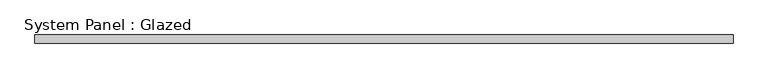
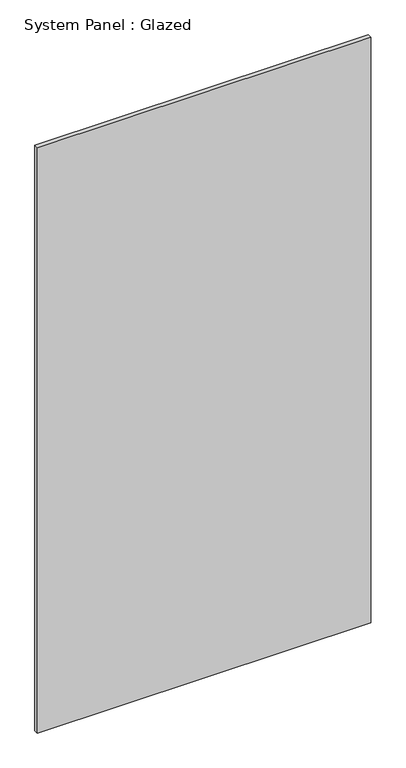
"""IFC4 building model written with IfcOpenShell, lengths in millimetres: plate geometry, System Panel : Glazed."""

from ifc_helpers import new_model, si_unit, origin, origin_with_axes, place, context, project, spatial, polyline, outline, extrude, source, transform, mapped, element, save


def system_panel_glazed_5d8041e7(model_context):
    return source(origin(), model_context, "Body", "SweptSolid", [
        extrude(outline(polyline([(1032.8813587, 19.05), (-1032.8813587, 19.05), (-1032.8813587, 44.45), (1032.8813587, 44.45), (1032.8813587, 19.05)])), origin_with_axes(), (0.0, 0.0, 1.0), 3835.4),
    ])


if __name__ == "__main__":
    model = new_model("IFC4")
    model_context = context("Model", 3, world=origin())
    ifc_project = project(units=[si_unit("LENGTHUNIT", "METRE", prefix="MILLI")], contexts=[model_context])
    site = spatial("IfcSite", under=ifc_project)
    building = spatial("IfcBuilding", under=site)
    placement = place(None, origin())
    system_panel_glazed_shape = system_panel_glazed_5d8041e7(model_context)
    element("IfcPlate", 1, ObjectType="System Panel : Glazed", at=placement, inside=building, context=model_context, shape_type="MappedRepresentation", body=[
        mapped(system_panel_glazed_shape, transform((0.0, 0.0, 0.0), x_axis=(1.0, 0.0, 0.0), y_axis=(0.0, 1.0, 0.0), z_axis=(0.0, 0.0, 1.0))),
    ])
    save(model, "model.ifc")

# Revit data of these elements
# Type "System Panel : Glazed"
#   Construction Type Id = "GSP4R"
#   Analytic Construction = "1/8 in Pilkington single glazing"
#   Visual Light Transmittance = 0.9
#   Solar Heat Gain Coefficient = 0.86
#   Heat Transfer Coefficient (U) = 1.18115 BTU/(h·ft²·°F)
# Element 1 (IfcPlate, "System Panel : Glazed")
#   Materials on its faces: "Glass"
# Materials
#   "Glass": class "Glass", colour RGB 0 128 192, transparency 0.75, Description = "Soda Lime Glass", Cost = 0
